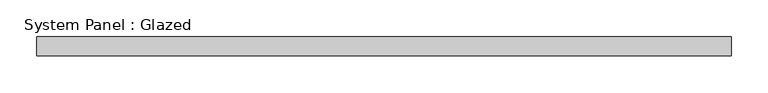
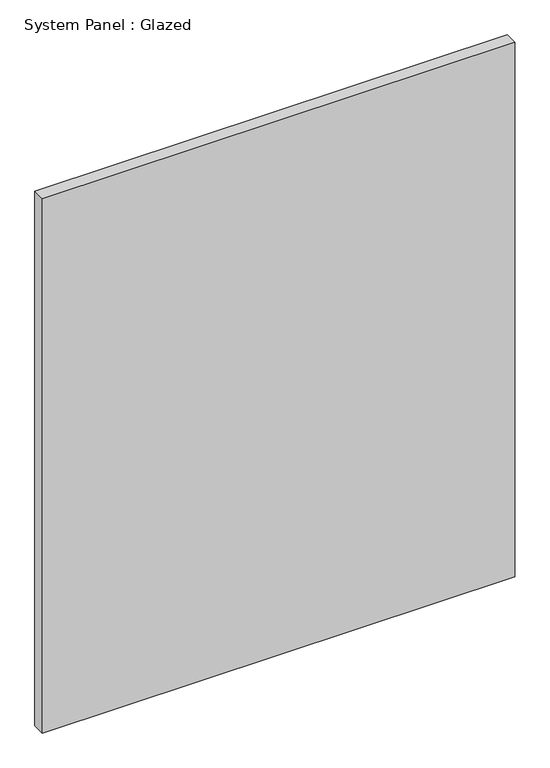
"""IFC4 building model written with IfcOpenShell, lengths in millimetres: plate geometry, System Panel : Glazed."""

from ifc_helpers import new_model, si_unit, origin, origin_with_axes, place, context, project, spatial, polyline, outline, extrude, source, transform, mapped, element, save


def system_panel_glazed_b6248f97(model_context):
    return source(origin(), model_context, "Body", "SweptSolid", [
        extrude(outline(polyline([(469.9, 19.05), (-469.9, 19.05), (-469.9, 44.45), (469.9, 44.45), (469.9, 19.05)])), origin_with_axes(), (0.0, 0.0, 1.0), 1123.95),
    ])


if __name__ == "__main__":
    model = new_model("IFC4")
    model_context = context("Model", 3, world=origin())
    ifc_project = project(units=[si_unit("LENGTHUNIT", "METRE", prefix="MILLI")], contexts=[model_context])
    site = spatial("IfcSite", under=ifc_project)
    building = spatial("IfcBuilding", under=site)
    placement = place(None, origin())
    system_panel_glazed_shape = system_panel_glazed_b6248f97(model_context)
    element("IfcPlate", 1, ObjectType="System Panel : Glazed", at=placement, inside=building, context=model_context, shape_type="MappedRepresentation", body=[
        mapped(system_panel_glazed_shape, transform((0.0, 0.0, 0.0), x_axis=(1.0, 0.0, 0.0), y_axis=(0.0, 1.0, 0.0), z_axis=(0.0, 0.0, 1.0))),
    ])
    save(model, "model.ifc")

# Revit data of these elements
# Type "System Panel : Glazed"
#   Construction Type Id = "GSP4R"
#   Analytic Construction = "1/8 in Pilkington single glazing"
#   Visual Light Transmittance = 0.9
#   Solar Heat Gain Coefficient = 0.86
#   Heat Transfer Coefficient (U) = 1.18115 BTU/(h·ft²·°F)
#   Define Thermal Properties by = 1
# Element 1 (IfcPlate, "System Panel : Glazed")
#   Materials on its faces: "Glass"
# Materials
#   "Glass": class "Glass", colour RGB 0 128 192, transparency 0.75, Description = "Soda Lime Glass", Cost = 0
